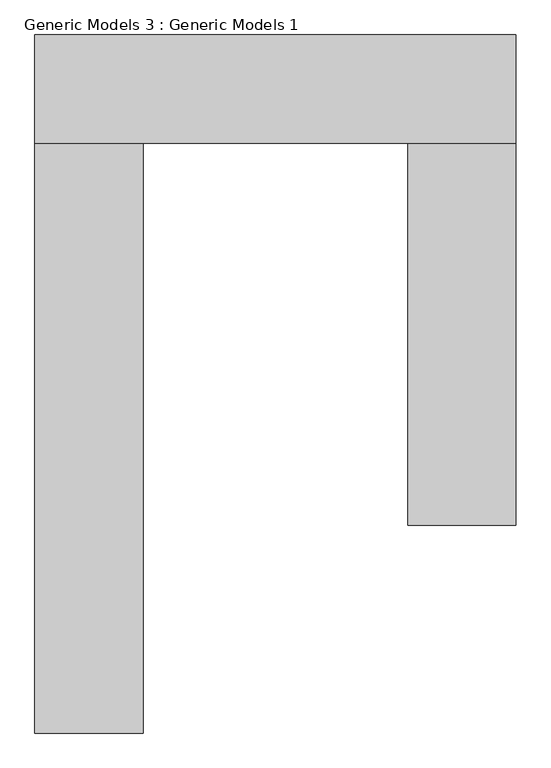
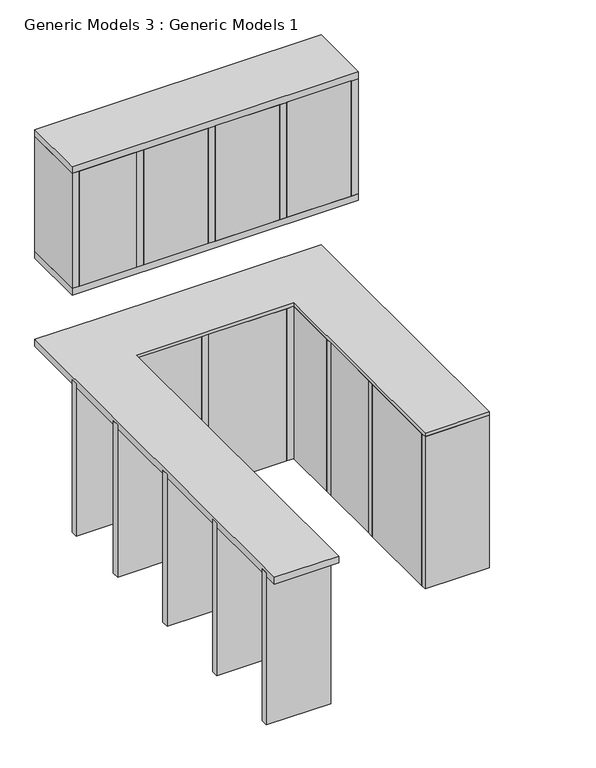
"""IFC4 building model written with IfcOpenShell, lengths in millimetres: proxy geometry, Generic Models 3 : Generic Models 1."""

from ifc_helpers import new_model, si_unit, frame, origin, place, context, project, spatial, polyline, outline, extrude, source, transform, mapped, element, save


def generic_models_3_generic_models_1_c5fb848b(model_context):
    return source(origin(), model_context, "Body", "SweptSolid", [
        extrude(outline(polyline([(-4007.5591227, 4416.7642852), (-4413.9591227, 4416.7642852), (-4413.9591227, 4436.1688715), (-4007.5591227, 4436.1688715), (-4007.5591227, 4416.7642852)])), frame((0.0, 0.0, 8280.4), z_axis=(0.0, 0.0, 1.0), x_axis=(1.0, 0.0, 0.0)), (0.0, 0.0, 1.0), 863.6),
        extrude(outline(polyline([(-3499.5591227, 4416.7642852), (-3956.7591227, 4416.7642852), (-3956.7591227, 4436.1688715), (-3499.5591227, 4436.1688715), (-3499.5591227, 4416.7642852)])), frame((0.0, 0.0, 8280.4), z_axis=(0.0, 0.0, 1.0), x_axis=(1.0, 0.0, 0.0)), (0.0, 0.0, 1.0), 863.6),
        extrude(outline(polyline([(-2991.5591227, 4416.7642852), (-3448.7591227, 4416.7642852), (-3448.7591227, 4436.1688715), (-2991.5591227, 4436.1688715), (-2991.5591227, 4416.7642852)])), frame((0.0, 0.0, 8280.4), z_axis=(0.0, 0.0, 1.0), x_axis=(1.0, 0.0, 0.0)), (0.0, 0.0, 1.0), 863.6),
        extrude(outline(polyline([(-2483.5591227, 4416.7642852), (-2940.7591227, 4416.7642852), (-2940.7591227, 4436.1688715), (-2483.5591227, 4436.1688715), (-2483.5591227, 4416.7642852)])), frame((0.0, 0.0, 8280.4), z_axis=(0.0, 0.0, 1.0), x_axis=(1.0, 0.0, 0.0)), (0.0, 0.0, 1.0), 863.6),
        extrude(outline(polyline([(-2432.7591227, 4873.9642852), (-2432.7591227, 4416.7642852), (-4464.7591227, 4416.7642852), (-4464.7591227, 4873.9642852), (-2432.7591227, 4873.9642852)])), frame((0.0, 0.0, 9144.0), z_axis=(0.0, 0.0, 1.0), x_axis=(1.0, 0.0, 0.0)), (0.0, 0.0, 1.0), 50.8),
        extrude(outline(polyline([(-4413.9591227, 4873.9642852), (-4413.9591227, 4416.7642852), (-4464.7591227, 4416.7642852), (-4464.7591227, 4873.9642852), (-4413.9591227, 4873.9642852)])), frame((0.0, 0.0, 8280.4), z_axis=(0.0, 0.0, 1.0), x_axis=(1.0, 0.0, 0.0)), (0.0, 0.0, 1.0), 863.6),
        extrude(outline(polyline([(-3956.7591227, 4873.9642852), (-3956.7591227, 4416.7642852), (-4007.5591227, 4416.7642852), (-4007.5591227, 4873.9642852), (-3956.7591227, 4873.9642852)])), frame((0.0, 0.0, 8280.4), z_axis=(0.0, 0.0, 1.0), x_axis=(1.0, 0.0, 0.0)), (0.0, 0.0, 1.0), 863.6),
        extrude(outline(polyline([(-3448.7591227, 4873.9642852), (-3448.7591227, 4416.7642852), (-3499.5591227, 4416.7642852), (-3499.5591227, 4873.9642852), (-3448.7591227, 4873.9642852)])), frame((0.0, 0.0, 8280.4), z_axis=(0.0, 0.0, 1.0), x_axis=(1.0, 0.0, 0.0)), (0.0, 0.0, 1.0), 863.6),
        extrude(outline(polyline([(-2991.5591227, 4873.9642852), (-2940.7591227, 4873.9642852), (-2940.7591227, 4416.7642852), (-2991.5591227, 4416.7642852), (-2991.5591227, 4873.9642852)])), frame((0.0, 0.0, 8280.4), z_axis=(0.0, 0.0, 1.0), x_axis=(1.0, 0.0, 0.0)), (0.0, 0.0, 1.0), 863.6),
        extrude(outline(polyline([(-2483.5591227, 4873.9642852), (-2432.7591227, 4873.9642852), (-2432.7591227, 4416.7642852), (-2483.5591227, 4416.7642852), (-2483.5591227, 4873.9642852)])), frame((0.0, 0.0, 8280.4), z_axis=(0.0, 0.0, 1.0), x_axis=(1.0, 0.0, 0.0)), (0.0, 0.0, 1.0), 863.6),
        extrude(outline(polyline([(-2432.7591227, 4873.9642852), (-2432.7591227, 4416.7642852), (-4464.7591227, 4416.7642852), (-4464.7591227, 4873.9642852), (-2432.7591227, 4873.9642852)])), frame((0.0, 0.0, 8229.6), z_axis=(0.0, 0.0, 1.0), x_axis=(1.0, 0.0, 0.0)), (0.0, 0.0, 1.0), 50.8),
        extrude(outline(polyline([(-4058.3591227, 2079.9642852), (-4058.3591227, 2638.7642852), (-4007.5591227, 2638.7642852), (-4007.5591227, 2079.9642852), (-4058.3591227, 2079.9642852)])), frame((0.0, 0.0, 6451.6), z_axis=(0.0, 0.0, 1.0), x_axis=(1.0, 0.0, 0.0)), (0.0, 0.0, 1.0), 1143.0),
        extrude(outline(polyline([(-4058.3591227, 2689.5642852), (-4058.3591227, 3248.3642852), (-4007.5591227, 3248.3642852), (-4007.5591227, 2689.5642852), (-4058.3591227, 2689.5642852)])), frame((0.0, 0.0, 6451.6), z_axis=(0.0, 0.0, 1.0), x_axis=(1.0, 0.0, 0.0)), (0.0, 0.0, 1.0), 1143.0),
        extrude(outline(polyline([(-4058.3591227, 3299.1642852), (-4058.3591227, 3857.9642852), (-4007.5591227, 3857.9642852), (-4007.5591227, 3299.1642852), (-4058.3591227, 3299.1642852)])), frame((0.0, 0.0, 6451.6), z_axis=(0.0, 0.0, 1.0), x_axis=(1.0, 0.0, 0.0)), (0.0, 0.0, 1.0), 1143.0),
        extrude(outline(polyline([(-4058.3591227, 3908.7642852), (-4058.3591227, 4365.9642852), (-4007.5591227, 4365.9642852), (-4007.5591227, 3908.7642852), (-4058.3591227, 3908.7642852)])), frame((0.0, 0.0, 6451.6), z_axis=(0.0, 0.0, 1.0), x_axis=(1.0, 0.0, 0.0)), (0.0, 0.0, 1.0), 1143.0),
        extrude(outline(polyline([(-4007.5591227, 4416.7642852), (-4007.5591227, 4455.5734579), (-3544.3461758, 4455.5734579), (-3544.3461758, 4416.7642852), (-4007.5591227, 4416.7642852)])), frame((0.0, 0.0, 6451.6), z_axis=(0.0, 0.0, 1.0), x_axis=(1.0, 0.0, 0.0)), (0.0, 0.0, 1.0), 1143.0),
        extrude(outline(polyline([(-3493.5461758, 4416.7642852), (-3493.5461758, 4455.5734579), (-2940.7591227, 4455.5734579), (-2940.7591227, 4416.7642852), (-3493.5461758, 4416.7642852)])), frame((0.0, 0.0, 6451.6), z_axis=(0.0, 0.0, 1.0), x_axis=(1.0, 0.0, 0.0)), (0.0, 0.0, 1.0), 1143.0),
        extrude(outline(polyline([(-2865.8793637, 4010.3642852), (-2889.9591227, 4010.3642852), (-2889.9591227, 4416.7642852), (-2865.8793637, 4416.7642852), (-2865.8793637, 4010.3642852)])), frame((0.0, 0.0, 6451.6), z_axis=(0.0, 0.0, 1.0), x_axis=(1.0, 0.0, 0.0)), (0.0, 0.0, 1.0), 1143.0),
        extrude(outline(polyline([(-2865.8793637, 3502.3642852), (-2889.9591227, 3502.3642852), (-2889.9591227, 3959.5642852), (-2865.8793637, 3959.5642852), (-2865.8793637, 3502.3642852)])), frame((0.0, 0.0, 6451.6), z_axis=(0.0, 0.0, 1.0), x_axis=(1.0, 0.0, 0.0)), (0.0, 0.0, 1.0), 1143.0),
        extrude(outline(polyline([(-2865.8793637, 2841.9642852), (-2889.9591227, 2841.9642852), (-2889.9591227, 3451.5642852), (-2865.8793637, 3451.5642852), (-2865.8793637, 2841.9642852)])), frame((0.0, 0.0, 6451.6), z_axis=(0.0, 0.0, 1.0), x_axis=(1.0, 0.0, 0.0)), (0.0, 0.0, 1.0), 1143.0),
        extrude(outline(polyline([(-4007.5591227, 2029.1642852), (-4464.7591227, 2029.1642852), (-4464.7591227, 2079.9642852), (-4007.5591227, 2079.9642852), (-4007.5591227, 2029.1642852)])), frame((0.0, 0.0, 6451.6), z_axis=(0.0, 0.0, 1.0), x_axis=(1.0, 0.0, 0.0)), (0.0, 0.0, 1.0), 1143.0),
        extrude(outline(polyline([(-4007.5591227, 2638.7642852), (-4464.7591227, 2638.7642852), (-4464.7591227, 2689.5642852), (-4007.5591227, 2689.5642852), (-4007.5591227, 2638.7642852)])), frame((0.0, 0.0, 6451.6), z_axis=(0.0, 0.0, 1.0), x_axis=(1.0, 0.0, 0.0)), (0.0, 0.0, 1.0), 1143.0),
        extrude(outline(polyline([(-4007.5591227, 3248.3642852), (-4464.7591227, 3248.3642852), (-4464.7591227, 3299.1642852), (-4007.5591227, 3299.1642852), (-4007.5591227, 3248.3642852)])), frame((0.0, 0.0, 6451.6), z_axis=(0.0, 0.0, 1.0), x_axis=(1.0, 0.0, 0.0)), (0.0, 0.0, 1.0), 1143.0),
        extrude(outline(polyline([(-4007.5591227, 3857.9642852), (-4464.7591227, 3857.9642852), (-4464.7591227, 3908.7642852), (-4007.5591227, 3908.7642852), (-4007.5591227, 3857.9642852)])), frame((0.0, 0.0, 6451.6), z_axis=(0.0, 0.0, 1.0), x_axis=(1.0, 0.0, 0.0)), (0.0, 0.0, 1.0), 1143.0),
        extrude(outline(polyline([(-4007.5591227, 4365.9642852), (-4464.7591227, 4365.9642852), (-4464.7591227, 4416.7642852), (-4007.5591227, 4416.7642852), (-4007.5591227, 4365.9642852)])), frame((0.0, 0.0, 6451.6), z_axis=(0.0, 0.0, 1.0), x_axis=(1.0, 0.0, 0.0)), (0.0, 0.0, 1.0), 1143.0),
        extrude(outline(polyline([(-3544.3461758, 4416.7642852), (-3544.3461758, 4873.9642852), (-3493.5461758, 4873.9642852), (-3493.5461758, 4416.7642852), (-3544.3461758, 4416.7642852)])), frame((0.0, 0.0, 6451.6), z_axis=(0.0, 0.0, 1.0), x_axis=(1.0, 0.0, 0.0)), (0.0, 0.0, 1.0), 1143.0),
        extrude(outline(polyline([(-2940.7591227, 4416.7642852), (-2940.7591227, 4873.9642852), (-2889.9591227, 4873.9642852), (-2889.9591227, 4416.7642852), (-2940.7591227, 4416.7642852)])), frame((0.0, 0.0, 6451.6), z_axis=(0.0, 0.0, 1.0), x_axis=(1.0, 0.0, 0.0)), (0.0, 0.0, 1.0), 1143.0),
        extrude(outline(polyline([(-2432.7591227, 2803.8642852), (-2889.9591227, 2803.8642852), (-2889.9591227, 2841.9642852), (-2432.7591227, 2841.9642852), (-2432.7591227, 2803.8642852)])), frame((0.0, 0.0, 6451.6), z_axis=(0.0, 0.0, 1.0), x_axis=(1.0, 0.0, 0.0)), (0.0, 0.0, 1.0), 1143.0),
        extrude(outline(polyline([(-2432.7591227, 3451.5642852), (-2889.9591227, 3451.5642852), (-2889.9591227, 3502.3642852), (-2432.7591227, 3502.3642852), (-2432.7591227, 3451.5642852)])), frame((0.0, 0.0, 6451.6), z_axis=(0.0, 0.0, 1.0), x_axis=(1.0, 0.0, 0.0)), (0.0, 0.0, 1.0), 1143.0),
        extrude(outline(polyline([(-2432.7591227, 3959.5642852), (-2889.9591227, 3959.5642852), (-2889.9591227, 4010.3642852), (-2432.7591227, 4010.3642852), (-2432.7591227, 3959.5642852)])), frame((0.0, 0.0, 6451.6), z_axis=(0.0, 0.0, 1.0), x_axis=(1.0, 0.0, 0.0)), (0.0, 0.0, 1.0), 1143.0),
        extrude(outline(polyline([(-4007.5591227, 1927.5642852), (-4464.7591227, 1927.5642852), (-4464.7591227, 4873.9642852), (-4008.5861775, 4873.9642852), (-2432.7591227, 4873.9642852), (-2432.7591227, 4519.1838129), (-2432.7591227, 2803.8642852), (-2889.9591227, 2803.8642852), (-2889.9591227, 4416.7642852), (-4007.5591227, 4416.7642852), (-4007.5591227, 1927.5642852)])), frame((0.0, 0.0, 7569.2), z_axis=(0.0, 0.0, 1.0), x_axis=(1.0, 0.0, 0.0)), (0.0, 0.0, 1.0), 50.8),
    ])


if __name__ == "__main__":
    model = new_model("IFC4")
    model_context = context("Model", 3, world=origin())
    ifc_project = project(units=[si_unit("LENGTHUNIT", "METRE", prefix="MILLI")], contexts=[model_context])
    site = spatial("IfcSite", under=ifc_project)
    building = spatial("IfcBuilding", under=site)
    placement = place(None, origin())
    generic_models_3_generic_models_1_shape = generic_models_3_generic_models_1_c5fb848b(model_context)
    element("IfcBuildingElementProxy", 1, Name="Generic Models 3 : Generic Models 1", ObjectType="Generic Models 3 : Generic Models 1", at=placement, inside=building, context=model_context, shape_type="MappedRepresentation", body=[
        mapped(generic_models_3_generic_models_1_shape, transform((0.0, 0.0, 0.0), x_axis=(1.0, 0.0, 0.0), y_axis=(0.0, 1.0, 0.0), z_axis=(0.0, 0.0, 1.0))),
    ])
    save(model, "model.ifc")
